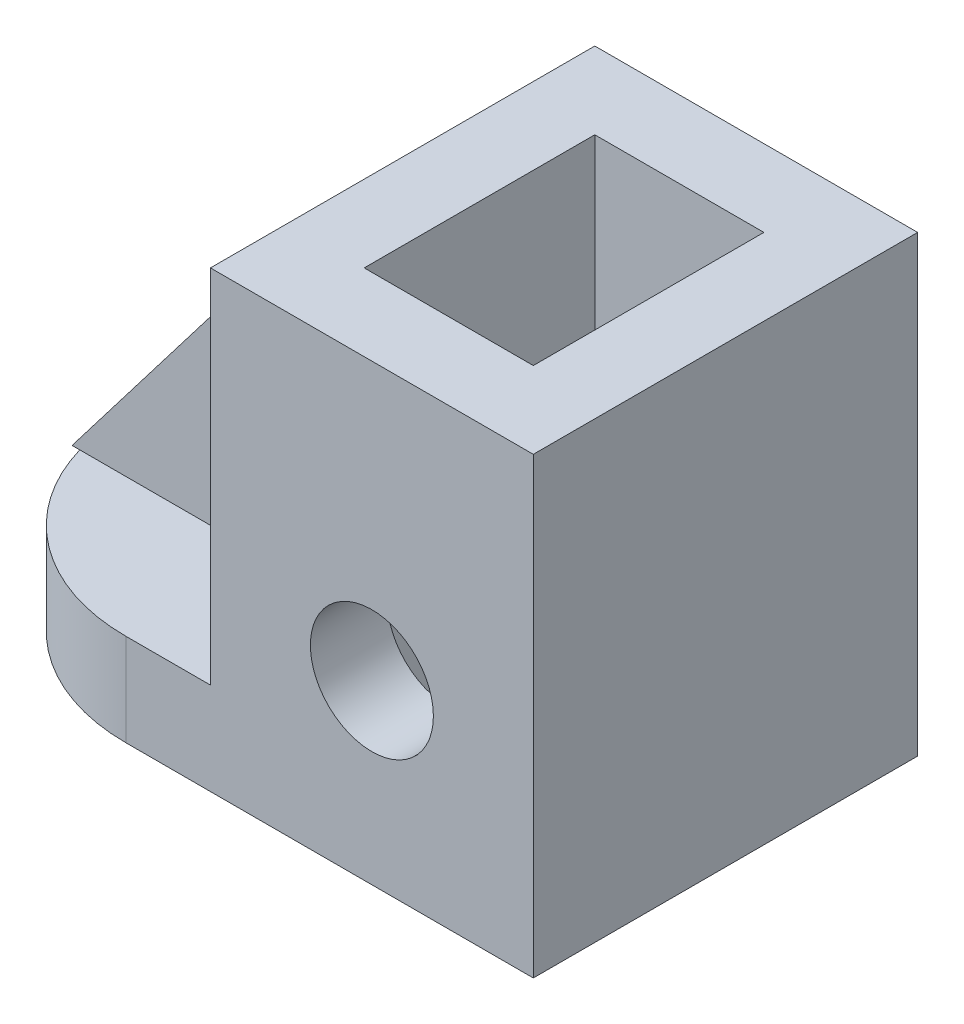
ISO-10303-21;
HEADER;
FILE_DESCRIPTION(('STEP AP214'),'2;1');
FILE_NAME('part.step','',(''),(''),'','','');
FILE_SCHEMA(('AUTOMOTIVE_DESIGN { 1 0 10303 214 1 1 1 1 }'));
ENDSEC;
DATA;
#1=APPLICATION_CONTEXT('core data for automotive mechanical design processes');
#2=APPLICATION_PROTOCOL_DEFINITION('international standard','automotive_design',2000,#1);
#3=PRODUCT_CONTEXT('',#1,'mechanical');
#4=PRODUCT('Part','Part','',(#3));
#5=PRODUCT_RELATED_PRODUCT_CATEGORY('part','',(#4));
#6=PRODUCT_DEFINITION_FORMATION('','',#4);
#7=PRODUCT_DEFINITION_CONTEXT('part definition',#1,'design');
#8=PRODUCT_DEFINITION('design','',#6,#7);
#9=PRODUCT_DEFINITION_SHAPE('','',#8);
#10=(LENGTH_UNIT() NAMED_UNIT(*) SI_UNIT(.MILLI.,.METRE.));
#11=(NAMED_UNIT(*) PLANE_ANGLE_UNIT() SI_UNIT($,.RADIAN.));
#12=(NAMED_UNIT(*) SI_UNIT($,.STERADIAN.) SOLID_ANGLE_UNIT());
#13=UNCERTAINTY_MEASURE_WITH_UNIT(LENGTH_MEASURE(1.E-05),#10,'distance_accuracy_value','');
#14=(GEOMETRIC_REPRESENTATION_CONTEXT(3) GLOBAL_UNCERTAINTY_ASSIGNED_CONTEXT((#13)) GLOBAL_UNIT_ASSIGNED_CONTEXT((#10,
#11,#12)) REPRESENTATION_CONTEXT('',''));
#15=CARTESIAN_POINT('',(0.,0.,0.));
#16=DIRECTION('',(0.,0.,1.));
#17=DIRECTION('',(1.,0.,0.));
#18=AXIS2_PLACEMENT_3D('',#15,#16,#17);
#19=CARTESIAN_POINT('',(0.,0.,0.));
#20=DIRECTION('',(0.,-1.,0.));
#21=DIRECTION('',(0.,0.,-1.));
#22=AXIS2_PLACEMENT_3D('',#19,#20,#21);
#23=PLANE('',#22);
#24=CARTESIAN_POINT('',(25.,0.,25.));
#25=DIRECTION('',(0.,1.,0.));
#26=DIRECTION('',(0.,0.,1.));
#27=AXIS2_PLACEMENT_3D('',#24,#25,#26);
#28=CIRCLE('',#27,25.);
#29=CARTESIAN_POINT('',(0.,0.,25.));
#30=VERTEX_POINT('',#29);
#31=CARTESIAN_POINT('',(0.99999999999998,0.,32.));
#32=VERTEX_POINT('',#31);
#33=EDGE_CURVE('E230',#30,#32,#28,.T.);
#34=ORIENTED_EDGE('',*,*,#33,.T.);
#35=DIRECTION('',(1.,0.,0.));
#36=VECTOR('',#35,1.);
#37=CARTESIAN_POINT('',(0.,0.,32.));
#38=LINE('',#37,#36);
#39=CARTESIAN_POINT('',(0.,0.,32.));
#40=VERTEX_POINT('',#39);
#41=EDGE_CURVE('E245',#40,#32,#38,.T.);
#42=ORIENTED_EDGE('',*,*,#41,.F.);
#43=DIRECTION('',(0.,0.,1.));
#44=VECTOR('',#43,1.);
#45=CARTESIAN_POINT('',(0.,0.,0.));
#46=LINE('',#45,#44);
#47=EDGE_CURVE('E243',#30,#40,#46,.T.);
#48=ORIENTED_EDGE('',*,*,#47,.F.);
#49=EDGE_LOOP('',(#34,#42,#48));
#50=FACE_BOUND('',#49,.T.);
#51=ADVANCED_FACE('F44',(#50),#23,.T.);
#52=CARTESIAN_POINT('',(36.,47.,0.));
#53=DIRECTION('',(-0.79387814600164,0.60807687778849,0.));
#54=DIRECTION('',(-0.60807687778849,-0.79387814600164,0.));
#55=AXIS2_PLACEMENT_3D('',#52,#53,#54);
#56=PLANE('',#55);
#57=DIRECTION('',(0.60807687778849,0.79387814600164,0.));
#58=VECTOR('',#57,1.);
#59=CARTESIAN_POINT('',(0.,0.,18.));
#60=LINE('',#59,#58);
#61=CARTESIAN_POINT('',(0.,0.,18.));
#62=VERTEX_POINT('',#61);
#63=CARTESIAN_POINT('',(36.,47.,18.));
#64=VERTEX_POINT('',#63);
#65=EDGE_CURVE('E159',#62,#64,#60,.T.);
#66=ORIENTED_EDGE('',*,*,#65,.F.);
#67=EDGE_CURVE('E251',#62,#30,#46,.T.);
#68=ORIENTED_EDGE('',*,*,#67,.T.);
#69=ORIENTED_EDGE('',*,*,#47,.T.);
#70=DIRECTION('',(-0.60807687778849,-0.79387814600164,0.));
#71=VECTOR('',#70,1.);
#72=CARTESIAN_POINT('',(36.,47.,32.));
#73=LINE('',#72,#71);
#74=CARTESIAN_POINT('',(36.,47.,32.));
#75=VERTEX_POINT('',#74);
#76=EDGE_CURVE('E166',#75,#40,#73,.T.);
#77=ORIENTED_EDGE('',*,*,#76,.F.);
#78=DIRECTION('',(0.,0.,1.));
#79=VECTOR('',#78,1.);
#80=CARTESIAN_POINT('',(36.,47.,50.));
#81=LINE('',#80,#79);
#82=EDGE_CURVE('E70',#64,#75,#81,.T.);
#83=ORIENTED_EDGE('',*,*,#82,.F.);
#84=EDGE_LOOP('',(#66,#68,#69,#77,#83));
#85=FACE_BOUND('',#84,.T.);
#86=ADVANCED_FACE('F168',(#85),#56,.T.);
#87=CARTESIAN_POINT('',(57.,11.,0.));
#88=DIRECTION('',(0.,0.,1.));
#89=DIRECTION('',(1.,0.,0.));
#90=AXIS2_PLACEMENT_3D('',#87,#88,#89);
#91=CYLINDRICAL_SURFACE('',#90,8.);
#92=CARTESIAN_POINT('',(57.,11.,10.));
#93=DIRECTION('',(0.,0.,-1.));
#94=DIRECTION('',(-1.,0.,0.));
#95=AXIS2_PLACEMENT_3D('',#92,#93,#94);
#96=CIRCLE('',#95,8.);
#97=CARTESIAN_POINT('',(49.,11.,10.));
#98=VERTEX_POINT('',#97);
#99=EDGE_CURVE('E197',#98,#98,#96,.F.);
#100=ORIENTED_EDGE('',*,*,#99,.T.);
#101=EDGE_LOOP('',(#100));
#102=FACE_BOUND('',#101,.T.);
#103=CARTESIAN_POINT('',(57.,11.,0.));
#104=DIRECTION('',(0.,0.,1.));
#105=DIRECTION('',(1.,0.,0.));
#106=AXIS2_PLACEMENT_3D('',#103,#104,#105);
#107=CIRCLE('',#106,8.);
#108=CARTESIAN_POINT('',(65.,11.,0.));
#109=VERTEX_POINT('',#108);
#110=EDGE_CURVE('E224',#109,#109,#107,.T.);
#111=ORIENTED_EDGE('',*,*,#110,.F.);
#112=EDGE_LOOP('',(#111));
#113=FACE_BOUND('',#112,.T.);
#114=ADVANCED_FACE('F303',(#102,#113),#91,.F.);
#115=CARTESIAN_POINT('',(78.,-12.,50.));
#116=DIRECTION('',(0.,1.,0.));
#117=DIRECTION('',(0.,0.,1.));
#118=AXIS2_PLACEMENT_3D('',#115,#116,#117);
#119=PLANE('',#118);
#120=DIRECTION('',(-1.,0.,0.));
#121=VECTOR('',#120,1.);
#122=CARTESIAN_POINT('',(78.,-12.,10.));
#123=LINE('',#122,#121);
#124=CARTESIAN_POINT('',(68.,-12.,10.));
#125=VERTEX_POINT('',#124);
#126=CARTESIAN_POINT('',(46.,-12.,10.));
#127=VERTEX_POINT('',#126);
#128=EDGE_CURVE('E201',#125,#127,#123,.T.);
#129=ORIENTED_EDGE('',*,*,#128,.T.);
#130=DIRECTION('',(0.,0.,1.));
#131=VECTOR('',#130,1.);
#132=CARTESIAN_POINT('',(46.,-12.,50.));
#133=LINE('',#132,#131);
#134=CARTESIAN_POINT('',(46.,-12.,40.));
#135=VERTEX_POINT('',#134);
#136=EDGE_CURVE('E216',#127,#135,#133,.T.);
#137=ORIENTED_EDGE('',*,*,#136,.T.);
#138=DIRECTION('',(1.,0.,0.));
#139=VECTOR('',#138,1.);
#140=CARTESIAN_POINT('',(78.,-12.,40.));
#141=LINE('',#140,#139);
#142=CARTESIAN_POINT('',(68.,-12.,40.));
#143=VERTEX_POINT('',#142);
#144=EDGE_CURVE('E196',#135,#143,#141,.T.);
#145=ORIENTED_EDGE('',*,*,#144,.T.);
#146=DIRECTION('',(0.,0.,-1.));
#147=VECTOR('',#146,1.);
#148=CARTESIAN_POINT('',(68.,-12.,50.));
#149=LINE('',#148,#147);
#150=EDGE_CURVE('E207',#143,#125,#149,.T.);
#151=ORIENTED_EDGE('',*,*,#150,.T.);
#152=EDGE_LOOP('',(#129,#137,#145,#151));
#153=FACE_BOUND('',#152,.T.);
#154=DIRECTION('',(1.,0.,0.));
#155=VECTOR('',#154,1.);
#156=CARTESIAN_POINT('',(78.,-12.,50.));
#157=LINE('',#156,#155);
#158=CARTESIAN_POINT('',(25.,-12.,50.));
#159=VERTEX_POINT('',#158);
#160=CARTESIAN_POINT('',(78.,-12.,50.));
#161=VERTEX_POINT('',#160);
#162=EDGE_CURVE('E190',#159,#161,#157,.T.);
#163=ORIENTED_EDGE('',*,*,#162,.F.);
#164=CARTESIAN_POINT('',(25.,-12.,25.));
#165=DIRECTION('',(0.,1.,0.));
#166=DIRECTION('',(0.,0.,1.));
#167=AXIS2_PLACEMENT_3D('',#164,#165,#166);
#168=CIRCLE('',#167,25.);
#169=CARTESIAN_POINT('',(25.,-12.,0.));
#170=VERTEX_POINT('',#169);
#171=EDGE_CURVE('E229',#170,#159,#168,.T.);
#172=ORIENTED_EDGE('',*,*,#171,.F.);
#173=DIRECTION('',(1.,0.,0.));
#174=VECTOR('',#173,1.);
#175=CARTESIAN_POINT('',(78.,-12.,0.));
#176=LINE('',#175,#174);
#177=CARTESIAN_POINT('',(78.,-12.,0.));
#178=VERTEX_POINT('',#177);
#179=EDGE_CURVE('E184',#170,#178,#176,.T.);
#180=ORIENTED_EDGE('',*,*,#179,.T.);
#181=DIRECTION('',(0.,0.,-1.));
#182=VECTOR('',#181,1.);
#183=CARTESIAN_POINT('',(78.,-12.,50.));
#184=LINE('',#183,#182);
#185=EDGE_CURVE('E52',#161,#178,#184,.T.);
#186=ORIENTED_EDGE('',*,*,#185,.F.);
#187=EDGE_LOOP('',(#163,#172,#180,#186));
#188=FACE_BOUND('',#187,.T.);
#189=ADVANCED_FACE('F50',(#153,#188),#119,.F.);
#190=CARTESIAN_POINT('',(0.,0.,50.));
#191=DIRECTION('',(0.,0.,-1.));
#192=DIRECTION('',(-1.,0.,0.));
#193=AXIS2_PLACEMENT_3D('',#190,#191,#192);
#194=PLANE('',#193);
#195=DIRECTION('',(1.,0.,0.));
#196=VECTOR('',#195,1.);
#197=CARTESIAN_POINT('',(36.,47.,50.));
#198=LINE('',#197,#196);
#199=CARTESIAN_POINT('',(36.,47.,50.));
#200=VERTEX_POINT('',#199);
#201=CARTESIAN_POINT('',(78.,47.,50.));
#202=VERTEX_POINT('',#201);
#203=EDGE_CURVE('E176',#200,#202,#198,.T.);
#204=ORIENTED_EDGE('',*,*,#203,.F.);
#205=DIRECTION('',(0.,1.,0.));
#206=VECTOR('',#205,1.);
#207=CARTESIAN_POINT('',(36.,47.,50.));
#208=LINE('',#207,#206);
#209=CARTESIAN_POINT('',(36.,0.,50.));
#210=VERTEX_POINT('',#209);
#211=EDGE_CURVE('E362',#210,#200,#208,.T.);
#212=ORIENTED_EDGE('',*,*,#211,.F.);
#213=DIRECTION('',(1.,0.,0.));
#214=VECTOR('',#213,1.);
#215=CARTESIAN_POINT('',(0.,0.,50.));
#216=LINE('',#215,#214);
#217=CARTESIAN_POINT('',(25.,0.,50.));
#218=VERTEX_POINT('',#217);
#219=EDGE_CURVE('E372',#218,#210,#216,.T.);
#220=ORIENTED_EDGE('',*,*,#219,.F.);
#221=DIRECTION('',(0.,1.,0.));
#222=VECTOR('',#221,1.);
#223=CARTESIAN_POINT('',(25.,-12.,50.));
#224=LINE('',#223,#222);
#225=EDGE_CURVE('E223',#159,#218,#224,.T.);
#226=ORIENTED_EDGE('',*,*,#225,.F.);
#227=ORIENTED_EDGE('',*,*,#162,.T.);
#228=DIRECTION('',(0.,1.,0.));
#229=VECTOR('',#228,1.);
#230=CARTESIAN_POINT('',(78.,0.,50.));
#231=LINE('',#230,#229);
#232=EDGE_CURVE('E186',#161,#202,#231,.T.);
#233=ORIENTED_EDGE('',*,*,#232,.T.);
#234=EDGE_LOOP('',(#204,#212,#220,#226,#227,#233));
#235=FACE_BOUND('',#234,.T.);
#236=CARTESIAN_POINT('',(57.,11.,50.));
#237=DIRECTION('',(0.,0.,1.));
#238=DIRECTION('',(1.,0.,0.));
#239=AXIS2_PLACEMENT_3D('',#236,#237,#238);
#240=CIRCLE('',#239,8.);
#241=CARTESIAN_POINT('',(65.,11.,50.));
#242=VERTEX_POINT('',#241);
#243=EDGE_CURVE('E217',#242,#242,#240,.T.);
#244=ORIENTED_EDGE('',*,*,#243,.F.);
#245=EDGE_LOOP('',(#244));
#246=FACE_BOUND('',#245,.T.);
#247=ADVANCED_FACE('F333',(#235,#246),#194,.F.);
#248=CARTESIAN_POINT('',(0.,0.,0.));
#249=DIRECTION('',(0.,0.,-1.));
#250=DIRECTION('',(-1.,0.,0.));
#251=AXIS2_PLACEMENT_3D('',#248,#249,#250);
#252=PLANE('',#251);
#253=DIRECTION('',(-1.,0.,0.));
#254=VECTOR('',#253,1.);
#255=CARTESIAN_POINT('',(36.,0.,0.));
#256=LINE('',#255,#254);
#257=CARTESIAN_POINT('',(36.,0.,0.));
#258=VERTEX_POINT('',#257);
#259=CARTESIAN_POINT('',(25.,0.,0.));
#260=VERTEX_POINT('',#259);
#261=EDGE_CURVE('E161',#258,#260,#256,.T.);
#262=ORIENTED_EDGE('',*,*,#261,.F.);
#263=DIRECTION('',(0.,-1.,0.));
#264=VECTOR('',#263,1.);
#265=CARTESIAN_POINT('',(36.,47.,0.));
#266=LINE('',#265,#264);
#267=CARTESIAN_POINT('',(36.,47.,0.));
#268=VERTEX_POINT('',#267);
#269=EDGE_CURVE('E365',#268,#258,#266,.T.);
#270=ORIENTED_EDGE('',*,*,#269,.F.);
#271=DIRECTION('',(1.,0.,0.));
#272=VECTOR('',#271,1.);
#273=CARTESIAN_POINT('',(36.,47.,0.));
#274=LINE('',#273,#272);
#275=CARTESIAN_POINT('',(78.,47.,0.));
#276=VERTEX_POINT('',#275);
#277=EDGE_CURVE('E174',#268,#276,#274,.T.);
#278=ORIENTED_EDGE('',*,*,#277,.T.);
#279=DIRECTION('',(0.,1.,0.));
#280=VECTOR('',#279,1.);
#281=CARTESIAN_POINT('',(78.,0.,0.));
#282=LINE('',#281,#280);
#283=EDGE_CURVE('E188',#178,#276,#282,.T.);
#284=ORIENTED_EDGE('',*,*,#283,.F.);
#285=ORIENTED_EDGE('',*,*,#179,.F.);
#286=DIRECTION('',(0.,1.,0.));
#287=VECTOR('',#286,1.);
#288=CARTESIAN_POINT('',(25.,-12.,0.));
#289=LINE('',#288,#287);
#290=EDGE_CURVE('E179',#170,#260,#289,.T.);
#291=ORIENTED_EDGE('',*,*,#290,.T.);
#292=EDGE_LOOP('',(#262,#270,#278,#284,#285,#291));
#293=FACE_BOUND('',#292,.T.);
#294=ORIENTED_EDGE('',*,*,#110,.T.);
#295=EDGE_LOOP('',(#294));
#296=FACE_BOUND('',#295,.T.);
#297=ADVANCED_FACE('F337',(#293,#296),#252,.T.);
#298=CARTESIAN_POINT('',(78.,0.,50.));
#299=DIRECTION('',(-1.,0.,0.));
#300=DIRECTION('',(0.,0.,1.));
#301=AXIS2_PLACEMENT_3D('',#298,#299,#300);
#302=PLANE('',#301);
#303=ORIENTED_EDGE('',*,*,#283,.T.);
#304=DIRECTION('',(0.,0.,1.));
#305=VECTOR('',#304,1.);
#306=CARTESIAN_POINT('',(78.,47.,50.));
#307=LINE('',#306,#305);
#308=EDGE_CURVE('E169',#276,#202,#307,.T.);
#309=ORIENTED_EDGE('',*,*,#308,.T.);
#310=ORIENTED_EDGE('',*,*,#232,.F.);
#311=ORIENTED_EDGE('',*,*,#185,.T.);
#312=EDGE_LOOP('',(#303,#309,#310,#311));
#313=FACE_BOUND('',#312,.T.);
#314=ADVANCED_FACE('F344',(#313),#302,.F.);
#315=CARTESIAN_POINT('',(36.,47.,50.));
#316=DIRECTION('',(0.,1.,0.));
#317=DIRECTION('',(0.,0.,1.));
#318=AXIS2_PLACEMENT_3D('',#315,#316,#317);
#319=PLANE('',#318);
#320=DIRECTION('',(0.,0.,1.));
#321=VECTOR('',#320,1.);
#322=CARTESIAN_POINT('',(46.,47.,10.));
#323=LINE('',#322,#321);
#324=CARTESIAN_POINT('',(46.,47.,10.));
#325=VERTEX_POINT('',#324);
#326=CARTESIAN_POINT('',(46.,47.,40.));
#327=VERTEX_POINT('',#326);
#328=EDGE_CURVE('E258',#325,#327,#323,.T.);
#329=ORIENTED_EDGE('',*,*,#328,.F.);
#330=DIRECTION('',(-1.,0.,0.));
#331=VECTOR('',#330,1.);
#332=CARTESIAN_POINT('',(46.,47.,10.));
#333=LINE('',#332,#331);
#334=CARTESIAN_POINT('',(68.,47.,10.));
#335=VERTEX_POINT('',#334);
#336=EDGE_CURVE('E270',#335,#325,#333,.T.);
#337=ORIENTED_EDGE('',*,*,#336,.F.);
#338=DIRECTION('',(0.,0.,-1.));
#339=VECTOR('',#338,1.);
#340=CARTESIAN_POINT('',(68.,47.,10.));
#341=LINE('',#340,#339);
#342=CARTESIAN_POINT('',(68.,47.,40.));
#343=VERTEX_POINT('',#342);
#344=EDGE_CURVE('E262',#343,#335,#341,.T.);
#345=ORIENTED_EDGE('',*,*,#344,.F.);
#346=DIRECTION('',(1.,0.,0.));
#347=VECTOR('',#346,1.);
#348=CARTESIAN_POINT('',(46.,47.,40.));
#349=LINE('',#348,#347);
#350=EDGE_CURVE('E265',#327,#343,#349,.T.);
#351=ORIENTED_EDGE('',*,*,#350,.F.);
#352=EDGE_LOOP('',(#329,#337,#345,#351));
#353=FACE_BOUND('',#352,.T.);
#354=ORIENTED_EDGE('',*,*,#308,.F.);
#355=ORIENTED_EDGE('',*,*,#277,.F.);
#356=EDGE_CURVE('E151',#268,#64,#81,.T.);
#357=ORIENTED_EDGE('',*,*,#356,.T.);
#358=ORIENTED_EDGE('',*,*,#82,.T.);
#359=DIRECTION('',(0.,0.,1.));
#360=VECTOR('',#359,1.);
#361=CARTESIAN_POINT('',(36.,47.,32.));
#362=LINE('',#361,#360);
#363=EDGE_CURVE('E255',#75,#200,#362,.T.);
#364=ORIENTED_EDGE('',*,*,#363,.T.);
#365=ORIENTED_EDGE('',*,*,#203,.T.);
#366=EDGE_LOOP('',(#354,#355,#357,#358,#364,#365));
#367=FACE_BOUND('',#366,.T.);
#368=ADVANCED_FACE('F173',(#353,#367),#319,.T.);
#369=CARTESIAN_POINT('',(25.,-12.,25.));
#370=DIRECTION('',(0.,1.,0.));
#371=DIRECTION('',(0.,0.,1.));
#372=AXIS2_PLACEMENT_3D('',#369,#370,#371);
#373=CYLINDRICAL_SURFACE('',#372,25.);
#374=CARTESIAN_POINT('',(0.99999999999998,0.,18.));
#375=VERTEX_POINT('',#374);
#376=EDGE_CURVE('E233',#260,#375,#28,.T.);
#377=ORIENTED_EDGE('',*,*,#376,.F.);
#378=ORIENTED_EDGE('',*,*,#290,.F.);
#379=ORIENTED_EDGE('',*,*,#171,.T.);
#380=ORIENTED_EDGE('',*,*,#225,.T.);
#381=CARTESIAN_POINT('',(25.,0.,25.));
#382=DIRECTION('',(0.,-1.,0.));
#383=DIRECTION('',(0.,0.,-1.));
#384=AXIS2_PLACEMENT_3D('',#381,#382,#383);
#385=CIRCLE('',#384,25.);
#386=EDGE_CURVE('E247',#32,#218,#385,.F.);
#387=ORIENTED_EDGE('',*,*,#386,.F.);
#388=ORIENTED_EDGE('',*,*,#33,.F.);
#389=EDGE_CURVE('E235',#375,#30,#28,.T.);
#390=ORIENTED_EDGE('',*,*,#389,.F.);
#391=EDGE_LOOP('',(#377,#378,#379,#380,#387,#388,#390));
#392=FACE_BOUND('',#391,.T.);
#393=ADVANCED_FACE('F250',(#392),#373,.T.);
#394=CARTESIAN_POINT('',(57.,11.,40.));
#395=DIRECTION('',(0.,0.,1.));
#396=DIRECTION('',(1.,0.,0.));
#397=AXIS2_PLACEMENT_3D('',#394,#395,#396);
#398=CIRCLE('',#397,8.);
#399=CARTESIAN_POINT('',(65.,11.,40.));
#400=VERTEX_POINT('',#399);
#401=EDGE_CURVE('E198',#400,#400,#398,.F.);
#402=ORIENTED_EDGE('',*,*,#401,.T.);
#403=EDGE_LOOP('',(#402));
#404=FACE_BOUND('',#403,.T.);
#405=ORIENTED_EDGE('',*,*,#243,.T.);
#406=EDGE_LOOP('',(#405));
#407=FACE_BOUND('',#406,.T.);
#408=ADVANCED_FACE('F295',(#404,#407),#91,.F.);
#409=CARTESIAN_POINT('',(46.,-33.,10.));
#410=DIRECTION('',(-1.,0.,0.));
#411=DIRECTION('',(0.,0.,1.));
#412=AXIS2_PLACEMENT_3D('',#409,#410,#411);
#413=PLANE('',#412);
#414=DIRECTION('',(0.,1.,0.));
#415=VECTOR('',#414,1.);
#416=CARTESIAN_POINT('',(46.,-33.,10.));
#417=LINE('',#416,#415);
#418=EDGE_CURVE('E199',#127,#325,#417,.T.);
#419=ORIENTED_EDGE('',*,*,#418,.T.);
#420=ORIENTED_EDGE('',*,*,#328,.T.);
#421=DIRECTION('',(0.,1.,0.));
#422=VECTOR('',#421,1.);
#423=CARTESIAN_POINT('',(46.,-33.,40.));
#424=LINE('',#423,#422);
#425=EDGE_CURVE('E211',#135,#327,#424,.T.);
#426=ORIENTED_EDGE('',*,*,#425,.F.);
#427=ORIENTED_EDGE('',*,*,#136,.F.);
#428=EDGE_LOOP('',(#419,#420,#426,#427));
#429=FACE_BOUND('',#428,.T.);
#430=ADVANCED_FACE('F292',(#429),#413,.F.);
#431=CARTESIAN_POINT('',(68.,-33.,10.));
#432=DIRECTION('',(1.,0.,0.));
#433=DIRECTION('',(0.,0.,-1.));
#434=AXIS2_PLACEMENT_3D('',#431,#432,#433);
#435=PLANE('',#434);
#436=DIRECTION('',(0.,1.,0.));
#437=VECTOR('',#436,1.);
#438=CARTESIAN_POINT('',(68.,-33.,40.));
#439=LINE('',#438,#437);
#440=EDGE_CURVE('E271',#143,#343,#439,.T.);
#441=ORIENTED_EDGE('',*,*,#440,.T.);
#442=ORIENTED_EDGE('',*,*,#344,.T.);
#443=DIRECTION('',(0.,1.,0.));
#444=VECTOR('',#443,1.);
#445=CARTESIAN_POINT('',(68.,-33.,10.));
#446=LINE('',#445,#444);
#447=EDGE_CURVE('E275',#125,#335,#446,.T.);
#448=ORIENTED_EDGE('',*,*,#447,.F.);
#449=ORIENTED_EDGE('',*,*,#150,.F.);
#450=EDGE_LOOP('',(#441,#442,#448,#449));
#451=FACE_BOUND('',#450,.T.);
#452=ADVANCED_FACE('F286',(#451),#435,.F.);
#453=CARTESIAN_POINT('',(46.,-33.,10.));
#454=DIRECTION('',(0.,0.,-1.));
#455=DIRECTION('',(-1.,0.,0.));
#456=AXIS2_PLACEMENT_3D('',#453,#454,#455);
#457=PLANE('',#456);
#458=ORIENTED_EDGE('',*,*,#99,.F.);
#459=EDGE_LOOP('',(#458));
#460=FACE_BOUND('',#459,.T.);
#461=ORIENTED_EDGE('',*,*,#447,.T.);
#462=ORIENTED_EDGE('',*,*,#336,.T.);
#463=ORIENTED_EDGE('',*,*,#418,.F.);
#464=ORIENTED_EDGE('',*,*,#128,.F.);
#465=EDGE_LOOP('',(#461,#462,#463,#464));
#466=FACE_BOUND('',#465,.T.);
#467=ADVANCED_FACE('F293',(#460,#466),#457,.F.);
#468=CARTESIAN_POINT('',(46.,-33.,40.));
#469=DIRECTION('',(0.,0.,1.));
#470=DIRECTION('',(1.,0.,0.));
#471=AXIS2_PLACEMENT_3D('',#468,#469,#470);
#472=PLANE('',#471);
#473=ORIENTED_EDGE('',*,*,#401,.F.);
#474=EDGE_LOOP('',(#473));
#475=FACE_BOUND('',#474,.T.);
#476=ORIENTED_EDGE('',*,*,#425,.T.);
#477=ORIENTED_EDGE('',*,*,#350,.T.);
#478=ORIENTED_EDGE('',*,*,#440,.F.);
#479=ORIENTED_EDGE('',*,*,#144,.F.);
#480=EDGE_LOOP('',(#476,#477,#478,#479));
#481=FACE_BOUND('',#480,.T.);
#482=ADVANCED_FACE('F278',(#475,#481),#472,.F.);
#483=DIRECTION('',(-1.,0.,0.));
#484=VECTOR('',#483,1.);
#485=CARTESIAN_POINT('',(0.,0.,18.));
#486=LINE('',#485,#484);
#487=EDGE_CURVE('E11',#375,#62,#486,.T.);
#488=ORIENTED_EDGE('',*,*,#487,.F.);
#489=ORIENTED_EDGE('',*,*,#389,.T.);
#490=ORIENTED_EDGE('',*,*,#67,.F.);
#491=EDGE_LOOP('',(#488,#489,#490));
#492=FACE_BOUND('',#491,.T.);
#493=ADVANCED_FACE('F310',(#492),#23,.T.);
#494=CARTESIAN_POINT('',(36.,47.,32.));
#495=DIRECTION('',(1.,0.,0.));
#496=DIRECTION('',(0.,0.,-1.));
#497=AXIS2_PLACEMENT_3D('',#494,#495,#496);
#498=PLANE('',#497);
#499=ORIENTED_EDGE('',*,*,#211,.T.);
#500=ORIENTED_EDGE('',*,*,#363,.F.);
#501=DIRECTION('',(0.,1.,0.));
#502=VECTOR('',#501,1.);
#503=CARTESIAN_POINT('',(36.,47.,32.));
#504=LINE('',#503,#502);
#505=CARTESIAN_POINT('',(36.,0.,32.));
#506=VERTEX_POINT('',#505);
#507=EDGE_CURVE('E377',#506,#75,#504,.T.);
#508=ORIENTED_EDGE('',*,*,#507,.F.);
#509=DIRECTION('',(0.,0.,1.));
#510=VECTOR('',#509,1.);
#511=CARTESIAN_POINT('',(36.,0.,32.));
#512=LINE('',#511,#510);
#513=EDGE_CURVE('E257',#506,#210,#512,.T.);
#514=ORIENTED_EDGE('',*,*,#513,.T.);
#515=EDGE_LOOP('',(#499,#500,#508,#514));
#516=FACE_BOUND('',#515,.T.);
#517=ADVANCED_FACE('F313',(#516),#498,.F.);
#518=CARTESIAN_POINT('',(0.,0.,32.));
#519=DIRECTION('',(0.,-1.,0.));
#520=DIRECTION('',(0.,0.,-1.));
#521=AXIS2_PLACEMENT_3D('',#518,#519,#520);
#522=PLANE('',#521);
#523=ORIENTED_EDGE('',*,*,#386,.T.);
#524=ORIENTED_EDGE('',*,*,#219,.T.);
#525=ORIENTED_EDGE('',*,*,#513,.F.);
#526=EDGE_CURVE('E376',#32,#506,#38,.T.);
#527=ORIENTED_EDGE('',*,*,#526,.F.);
#528=EDGE_LOOP('',(#523,#524,#525,#527));
#529=FACE_BOUND('',#528,.T.);
#530=ADVANCED_FACE('F322',(#529),#522,.F.);
#531=CARTESIAN_POINT('',(0.,0.,32.));
#532=DIRECTION('',(0.,0.,1.));
#533=DIRECTION('',(1.,0.,0.));
#534=AXIS2_PLACEMENT_3D('',#531,#532,#533);
#535=PLANE('',#534);
#536=ORIENTED_EDGE('',*,*,#76,.T.);
#537=ORIENTED_EDGE('',*,*,#41,.T.);
#538=ORIENTED_EDGE('',*,*,#526,.T.);
#539=ORIENTED_EDGE('',*,*,#507,.T.);
#540=EDGE_LOOP('',(#536,#537,#538,#539));
#541=FACE_BOUND('',#540,.T.);
#542=ADVANCED_FACE('F383',(#541),#535,.T.);
#543=CARTESIAN_POINT('',(36.,0.,18.));
#544=DIRECTION('',(0.,-1.,0.));
#545=DIRECTION('',(0.,0.,-1.));
#546=AXIS2_PLACEMENT_3D('',#543,#544,#545);
#547=PLANE('',#546);
#548=ORIENTED_EDGE('',*,*,#376,.T.);
#549=DIRECTION('',(-1.,0.,0.));
#550=VECTOR('',#549,1.);
#551=CARTESIAN_POINT('',(36.,0.,18.));
#552=LINE('',#551,#550);
#553=CARTESIAN_POINT('',(36.,0.,18.));
#554=VERTEX_POINT('',#553);
#555=EDGE_CURVE('E56',#554,#375,#552,.T.);
#556=ORIENTED_EDGE('',*,*,#555,.F.);
#557=DIRECTION('',(0.,0.,-1.));
#558=VECTOR('',#557,1.);
#559=CARTESIAN_POINT('',(36.,0.,18.));
#560=LINE('',#559,#558);
#561=EDGE_CURVE('E152',#554,#258,#560,.T.);
#562=ORIENTED_EDGE('',*,*,#561,.T.);
#563=ORIENTED_EDGE('',*,*,#261,.T.);
#564=EDGE_LOOP('',(#548,#556,#562,#563));
#565=FACE_BOUND('',#564,.T.);
#566=ADVANCED_FACE('F387',(#565),#547,.F.);
#567=CARTESIAN_POINT('',(36.,47.,18.));
#568=DIRECTION('',(1.,0.,0.));
#569=DIRECTION('',(0.,0.,-1.));
#570=AXIS2_PLACEMENT_3D('',#567,#568,#569);
#571=PLANE('',#570);
#572=ORIENTED_EDGE('',*,*,#269,.T.);
#573=ORIENTED_EDGE('',*,*,#561,.F.);
#574=DIRECTION('',(0.,-1.,0.));
#575=VECTOR('',#574,1.);
#576=CARTESIAN_POINT('',(36.,47.,18.));
#577=LINE('',#576,#575);
#578=EDGE_CURVE('E146',#64,#554,#577,.T.);
#579=ORIENTED_EDGE('',*,*,#578,.F.);
#580=ORIENTED_EDGE('',*,*,#356,.F.);
#581=EDGE_LOOP('',(#572,#573,#579,#580));
#582=FACE_BOUND('',#581,.T.);
#583=ADVANCED_FACE('F155',(#582),#571,.F.);
#584=CARTESIAN_POINT('',(0.,0.,18.));
#585=DIRECTION('',(0.,0.,1.));
#586=DIRECTION('',(1.,0.,0.));
#587=AXIS2_PLACEMENT_3D('',#584,#585,#586);
#588=PLANE('',#587);
#589=ORIENTED_EDGE('',*,*,#65,.T.);
#590=ORIENTED_EDGE('',*,*,#578,.T.);
#591=ORIENTED_EDGE('',*,*,#555,.T.);
#592=ORIENTED_EDGE('',*,*,#487,.T.);
#593=EDGE_LOOP('',(#589,#590,#591,#592));
#594=FACE_BOUND('',#593,.T.);
#595=ADVANCED_FACE('F158',(#594),#588,.F.);
#596=CLOSED_SHELL('',(#51,#86,#114,#189,#247,#297,#314,#368,#393,#408,#430,#452,#467,#482,#493,
#517,#530,#542,#566,#583,#595));
#597=MANIFOLD_SOLID_BREP('B2',#596);
#598=ADVANCED_BREP_SHAPE_REPRESENTATION('',(#18,#597),#14);
#599=SHAPE_DEFINITION_REPRESENTATION(#9,#598);
ENDSEC;
END-ISO-10303-21;
